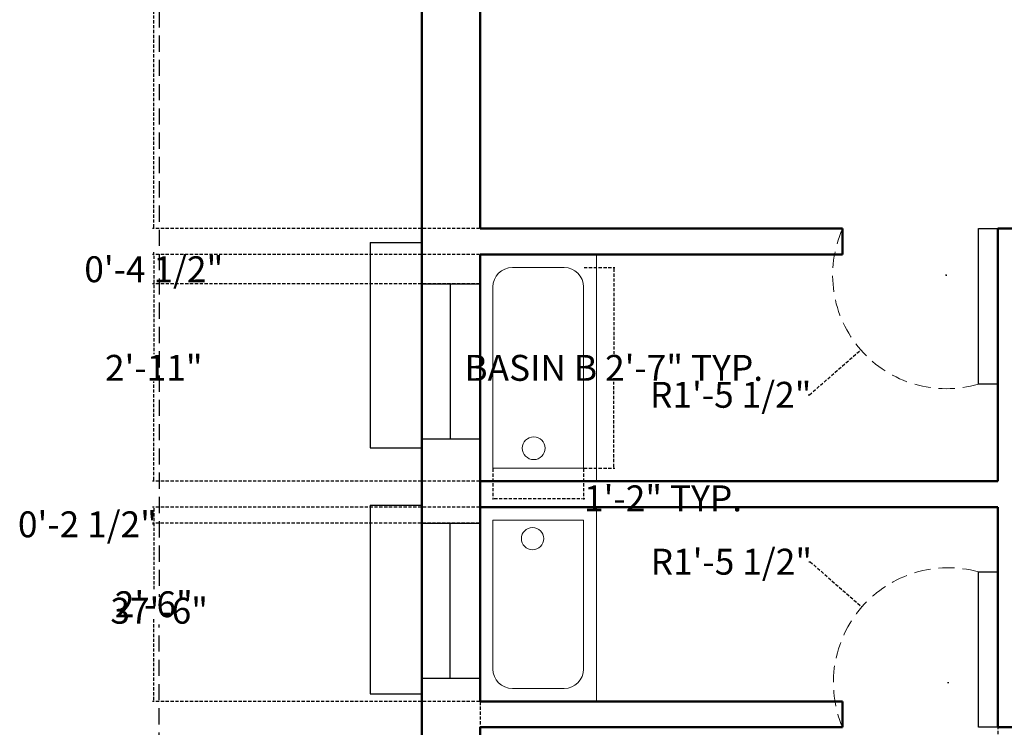
# Model space of a CAD drawing. Units: inches. Extents: x 513 to 1142, y 396 to 927.
# Tile 3 of 31: x 513 to 665, y 637 to 746. Entities that reach past the tile are written whole.
import ezdxf

# ---------------------------------------------------------------- set-up
doc = ezdxf.new("R2010")
doc.units = ezdxf.units.IN
doc.header["$MEASUREMENT"] = 0
doc.linetypes.add('DASHED', pattern=[0.75, 0.5, -0.25])
for name, color, linetype, lineweight in [('A-ANNO-DIMS', 2, 'DASHED', 18), ('A-DOOR', 4, 'Continuous', 25), ('A-DOOR-SWNG', 4, 'DASHED', 13), ('A-FLOR-FIXT', 92, 'Continuous', 18), ('A-WALL', 7, 'Continuous', 50), ('windows', 172, 'Continuous', 25)]:
    doc.layers.add(name, color=color, linetype=linetype, lineweight=lineweight)
doc.styles.get("Standard").update_dxf_attribs({"font": 'arial.ttf'})
doc.dimstyles.get("Standard").update_dxf_attribs({"dimtxt": 4, "dimasz": 0.18, "dimexe": 0.18, "dimexo": 0.0625, "dimgap": 0.09, "dimtad": 0, "dimtih": 1, "dimtoh": 1, "dimdec": 0, "dimrnd": 6, "dimzin": 0, "dimdsep": 46, "dimlunit": 3, "dimtxsty": 'Standard', "dimcen": 0.09, "dimadec": 0, "dimazin": 0, "dimtfac": 1, "dimtdec": 0, "dimtofl": 0, "dimtmove": 0, "dimatfit": 3, "dimfxl": 1, "dimtolj": 1, "dimtzin": 0, "dimarcsym": 0})

# ---------------------------------------------------------------- blocks, each defined once
blk = doc.blocks.new('*D104')
at = {"layer": 'A-ANNO-DIMS', "color": 0, "lineweight": -2, "ltscale": 5, "transparency": 16777216}
for p, q in [((574.93, 879.16), (534.25, 879.16)), ((534.43, 878.98), (534.43, 657.29)), ((534.43, 431.34), (534.43, 653.02)), ((574.93, 431.16), (534.25, 431.16))]:
    blk.add_line(p, q, dxfattribs=at)
at = {"layer": 'A-ANNO-DIMS', "color": 0, "ltscale": 5, "transparency": 16777216}
for points in [[(534.4, 878.98), (534.46, 878.98), (534.43, 879.16)], [(534.4, 431.34), (534.46, 431.34), (534.43, 431.16)]]:
    blk.add_solid(points, dxfattribs=at)
at = {"layer": 'Defpoints', "color": 0, "ltscale": 5, "transparency": 16777216}
for p in [(575, 879.16), (534.43, 431.16), (575, 431.16)]:
    blk.add_point(p, dxfattribs=at)
at = {"layer": 'A-ANNO-DIMS', "color": 0, "ltscale": 5, "transparency": 16777216, "insert": (534.43, 655.16), "char_height": 4, "attachment_point": 5}
blk.add_mtext('\\A1;37\'-6"', dxfattribs=at)
blk = doc.blocks.new('WIN-24IN')
blk.add_line((0, 4.39), (24, 4.39))
blk.add_lwpolyline([(24, 0), (0, 0), (0, 9), (24, 9)], close=True)
blk = doc.blocks.new('DOOR-LEAF-24IN')
blk.add_lwpolyline([(3, 24), (3, 0), (0, 0), (0, 24)], close=True)
blk = doc.blocks.new('BASIN-BOWL-14X26')
for p, q in [((0, 3), (0, 26)), ((0, 26), (14, 26)), ((14, 3), (14, 26)), ((3, 0), (11, 0))]:
    blk.add_line(p, q)
for centre, start, end in [((3, 3), 180, 270), ((11, 3), 270, 0)]:
    blk.add_arc(centre, 3, start, end)
blk = doc.blocks.new('BASIN-BOWL-14X31')
for p, q in [((11, 31), (3, 31)), ((0, 0), (0, 28)), ((14, 0), (14, 28)), ((0, 0), (14, 0))]:
    blk.add_line(p, q)
for centre, start, end in [((3, 28), 90, 180), ((11, 28), 0, 90)]:
    blk.add_arc(centre, 3, start, end)
blk = doc.blocks.new('*D133')
at = {"layer": 'A-ANNO-DIMS', "color": 0, "lineweight": -2, "transparency": 16777216}
for p, q in [((600.06, 708.16), (604.83, 708.16)), ((604.65, 707.98), (604.65, 694.82)), ((604.65, 677.34), (604.65, 690.5)), ((600.06, 677.16), (604.83, 677.16))]:
    blk.add_line(p, q, dxfattribs=at)
at = {"layer": 'A-ANNO-DIMS', "color": 0, "transparency": 16777216}
for points in [[(604.62, 707.98), (604.68, 707.98), (604.65, 708.16)], [(604.62, 677.34), (604.68, 677.34), (604.65, 677.16)]]:
    blk.add_solid(points, dxfattribs=at)
at = {"layer": 'Defpoints', "color": 0, "transparency": 16777216}
for p in [(600, 708.16), (604.65, 708.16), (600, 677.16)]:
    blk.add_point(p, dxfattribs=at)
at = {"layer": 'A-ANNO-DIMS', "color": 0, "transparency": 16777216, "insert": (604.65, 692.66), "char_height": 4, "attachment_point": 5}
blk.add_mtext('\\A1;BASIN B 2\'-7" TYP.', dxfattribs=at)
blk = doc.blocks.new('*D134')
at = {"layer": 'A-ANNO-DIMS', "color": 0, "lineweight": -2, "transparency": 16777216}
for p, q in [((586, 677.1), (586, 672.33)), ((600, 677.1), (600, 672.33)), ((586.18, 672.51), (599.82, 672.51)), ((600, 672.51), (600.18, 672.51))]:
    blk.add_line(p, q, dxfattribs=at)
at = {"layer": 'A-ANNO-DIMS', "color": 0, "transparency": 16777216}
for points in [[(586.18, 672.54), (586.18, 672.48), (586, 672.51)], [(599.82, 672.54), (599.82, 672.48), (600, 672.51)]]:
    blk.add_solid(points, dxfattribs=at)
at = {"layer": 'Defpoints', "color": 0, "transparency": 16777216}
for p in [(586, 677.16), (600, 677.16), (600, 672.51)]:
    blk.add_point(p, dxfattribs=at)
at = {"layer": 'A-ANNO-DIMS', "color": 0, "transparency": 16777216, "insert": (612.27, 672.51), "char_height": 4, "attachment_point": 5}
blk.add_mtext('\\A1;1\'-2" TYP.', dxfattribs=at)
blk = doc.blocks.new('*D139')
at = {"layer": 'A-ANNO-DIMS', "color": 0, "lineweight": -2, "transparency": 16777216}
for p, q in [((583.93, 870.16), (533.42, 870.16)), ((533.6, 869.98), (533.6, 794.29)), ((533.6, 714.34), (533.6, 790.02)), ((583.93, 714.16), (533.42, 714.16))]:
    blk.add_line(p, q, dxfattribs=at)
at = {"layer": 'A-ANNO-DIMS', "color": 0, "transparency": 16777216}
for points in [[(533.57, 869.98), (533.63, 869.98), (533.6, 870.16)], [(533.57, 714.34), (533.63, 714.34), (533.6, 714.16)]]:
    blk.add_solid(points, dxfattribs=at)
at = {"layer": 'Defpoints', "color": 0, "transparency": 16777216}
for p in [(533.6, 870.16), (584, 870.16), (584, 714.16)]:
    blk.add_point(p, dxfattribs=at)
at = {"layer": 'A-ANNO-DIMS', "color": 0, "transparency": 16777216, "insert": (533.6, 792.16), "char_height": 4, "attachment_point": 5}
blk.add_mtext('\\A1;13\'-0"', dxfattribs=at)
blk = doc.blocks.new('*D140')
at = {"layer": 'A-ANNO-DIMS', "color": 0, "lineweight": -2, "transparency": 16777216}
for p, q in [((583.93, 710.16), (533.42, 710.16)), ((533.6, 709.98), (533.6, 694.76)), ((533.6, 675.34), (533.6, 690.56)), ((583.93, 675.16), (533.42, 675.16))]:
    blk.add_line(p, q, dxfattribs=at)
at = {"layer": 'A-ANNO-DIMS', "color": 0, "transparency": 16777216}
for points in [[(533.57, 709.98), (533.63, 709.98), (533.6, 710.16)], [(533.57, 675.34), (533.63, 675.34), (533.6, 675.16)]]:
    blk.add_solid(points, dxfattribs=at)
at = {"layer": 'Defpoints', "color": 0, "transparency": 16777216}
for p in [(533.6, 710.16), (584, 710.16), (584, 675.16)]:
    blk.add_point(p, dxfattribs=at)
at = {"layer": 'A-ANNO-DIMS', "color": 0, "transparency": 16777216, "insert": (533.6, 692.66), "char_height": 4, "attachment_point": 5}
blk.add_mtext('\\A1;2\'-11"', dxfattribs=at)
blk = doc.blocks.new('*D141')
at = {"layer": 'A-ANNO-DIMS', "color": 0, "lineweight": -2, "transparency": 16777216}
for p, q in [((583.93, 671.16), (533.42, 671.16)), ((533.6, 670.98), (533.6, 658.29)), ((533.6, 641.34), (533.6, 654.03)), ((583.93, 641.16), (533.42, 641.16))]:
    blk.add_line(p, q, dxfattribs=at)
at = {"layer": 'A-ANNO-DIMS', "color": 0, "transparency": 16777216}
for points in [[(533.57, 670.98), (533.63, 670.98), (533.6, 671.16)], [(533.57, 641.34), (533.63, 641.34), (533.6, 641.16)]]:
    blk.add_solid(points, dxfattribs=at)
at = {"layer": 'Defpoints', "color": 0, "transparency": 16777216}
for p in [(533.6, 671.16), (584, 671.16), (584, 641.16)]:
    blk.add_point(p, dxfattribs=at)
at = {"layer": 'A-ANNO-DIMS', "color": 0, "transparency": 16777216, "insert": (533.6, 656.16), "char_height": 4, "attachment_point": 5}
blk.add_mtext('\\A1;2\'-6"', dxfattribs=at)
blk = doc.blocks.new('*D147')
at = {"layer": 'A-ANNO-DIMS', "color": 0, "lineweight": -2, "transparency": 16777216}
for p, q in [((584, 671.1), (584, 401.58)), ((664, 671.1), (664, 401.58)), ((584.18, 401.76), (618.58, 401.76)), ((663.82, 401.76), (629.41, 401.76))]:
    blk.add_line(p, q, dxfattribs=at)
at = {"layer": 'A-ANNO-DIMS', "color": 0, "transparency": 16777216}
for points in [[(584.18, 401.79), (584.18, 401.73), (584, 401.76)], [(663.82, 401.79), (663.82, 401.73), (664, 401.76)]]:
    blk.add_solid(points, dxfattribs=at)
at = {"layer": 'Defpoints', "color": 0, "transparency": 16777216}
for p in [(584, 671.16), (664, 671.16), (664, 401.76)]:
    blk.add_point(p, dxfattribs=at)
at = {"layer": 'A-ANNO-DIMS', "color": 0, "transparency": 16777216, "insert": (624, 401.76), "char_height": 4, "attachment_point": 5}
blk.add_mtext('\\A1;6\'-8"', dxfattribs=at)
blk = doc.blocks.new('*D163')
at = {"layer": 'A-ANNO-DIMS', "color": 0, "lineweight": -2, "transparency": 16777216}
for p, q in [((533.6, 710.34), (533.6, 710.52)), ((583.93, 710.16), (533.42, 710.16)), ((583.94, 705.63), (533.42, 705.63)), ((533.6, 705.45), (533.6, 705.27))]:
    blk.add_line(p, q, dxfattribs=at)
at = {"layer": 'A-ANNO-DIMS', "color": 0, "transparency": 16777216}
for points in [[(533.57, 710.34), (533.63, 710.34), (533.6, 710.16)], [(533.57, 705.45), (533.63, 705.45), (533.6, 705.63)]]:
    blk.add_solid(points, dxfattribs=at)
at = {"layer": 'Defpoints', "color": 0, "transparency": 16777216}
for p in [(584, 710.16), (533.6, 705.63), (584.01, 705.63)]:
    blk.add_point(p, dxfattribs=at)
at = {"layer": 'A-ANNO-DIMS', "color": 0, "transparency": 16777216, "insert": (533.6, 707.89), "char_height": 4, "attachment_point": 5}
blk.add_mtext('\\A1;0\'-4 1/2"', dxfattribs=at)
blk = doc.blocks.new('*D164')
at = {"layer": 'A-ANNO-DIMS', "color": 0, "lineweight": -2, "transparency": 16777216}
for p, q in [((583.93, 671.16), (533.42, 671.16)), ((533.6, 670.98), (533.6, 668.86)), ((583.89, 668.68), (533.42, 668.68)), ((533.6, 668.5), (533.42, 668.5)), ((533.6, 668.68), (533.6, 668.5))]:
    blk.add_line(p, q, dxfattribs=at)
at = {"layer": 'A-ANNO-DIMS', "color": 0, "transparency": 16777216}
for points in [[(533.57, 670.98), (533.63, 670.98), (533.6, 671.16)], [(533.57, 668.86), (533.63, 668.86), (533.6, 668.68)]]:
    blk.add_solid(points, dxfattribs=at)
at = {"layer": 'Defpoints', "color": 0, "transparency": 16777216}
for p in [(584, 671.16), (533.6, 668.68), (583.95, 668.68)]:
    blk.add_point(p, dxfattribs=at)
at = {"layer": 'A-ANNO-DIMS', "color": 0, "transparency": 16777216, "insert": (523.35, 668.5), "char_height": 4, "attachment_point": 5}
blk.add_mtext('\\A1;0\'-2 1/2"', dxfattribs=at)
blk = doc.blocks.new('*D187')
at = {"layer": 'A-ANNO-DIMS', "color": 0, "lineweight": -2, "transparency": 16777216}
for p, q in [((634.8, 662.73), (634.98, 662.73)), ((634.98, 662.73), (642.85, 655.85)), ((656.23, 644.06), (656.41, 644.06)), ((656.32, 643.97), (656.32, 644.15))]:
    blk.add_line(p, q, dxfattribs=at)
at = {"layer": 'A-ANNO-DIMS', "color": 0, "transparency": 16777216}
blk.add_solid([(642.87, 655.87), (642.83, 655.83), (642.98, 655.73)], dxfattribs=at)
at = {"layer": 'Defpoints', "color": 0, "transparency": 16777216}
for p in [(642.98, 655.73), (656.32, 644.06)]:
    blk.add_point(p, dxfattribs=at)
at = {"layer": 'A-ANNO-DIMS', "color": 0, "transparency": 16777216, "insert": (622.82, 662.73), "char_height": 4, "attachment_point": 5}
blk.add_mtext('\\A1;R1\'-5 1/2"', dxfattribs=at)
blk = doc.blocks.new('*D188')
at = {"layer": 'A-ANNO-DIMS', "color": 0, "lineweight": -2, "transparency": 16777216}
for p, q in [((655.93, 706.99), (656.11, 706.99)), ((656.02, 706.9), (656.02, 707.08)), ((634.88, 688.5), (642.67, 695.32)), ((634.7, 688.5), (634.88, 688.5))]:
    blk.add_line(p, q, dxfattribs=at)
at = {"layer": 'A-ANNO-DIMS', "color": 0, "transparency": 16777216}
blk.add_solid([(642.65, 695.34), (642.69, 695.29), (642.81, 695.43)], dxfattribs=at)
at = {"layer": 'Defpoints', "color": 0, "transparency": 16777216}
for p in [(656.02, 706.99), (642.81, 695.43)]:
    blk.add_point(p, dxfattribs=at)
at = {"layer": 'A-ANNO-DIMS', "color": 0, "transparency": 16777216, "insert": (622.72, 688.5), "char_height": 4, "attachment_point": 5}
blk.add_mtext('\\A1;R1\'-5 1/2"', dxfattribs=at)

msp = doc.modelspace()

# ---------------------------------------------------------------- linework, layer by layer
at = {"layer": 'A-DOOR-SWNG', "ltscale": 5}
for centre, radius, start, end in [((656.02, 706.99), 17.55, 155.9122, 286.4597), ((656.32, 644.06), 17.73, 74.72, 202.9082)]:
    msp.add_arc(centre, radius, start, end, dxfattribs=at)
at = {"layer": 'A-FLOR-FIXT'}
for p, q in [((602, 710.16), (602, 675.16)), ((602, 671.16), (602, 641.16))]:
    msp.add_line(p, q, dxfattribs=at)
for centre, radius in [((592.29, 680.26), 1.76), ((592.11, 666.29), 1.72)]:
    msp.add_circle(centre, radius, dxfattribs=at)
at = {"layer": 'A-WALL'}
for p, q in [((575, 879.16), (575, 431.16)), ((584, 870.16), (584, 714.16)), ((640, 714.16), (584, 714.16)), ((640, 714.16), (640, 710.16)), ((704, 714.16), (664, 714.16)), ((664, 714.16), (664, 675.16)), ((640, 710.16), (584, 710.16)), ((584, 710.16), (584, 641.16)), ((584, 675.16), (664, 675.16)), ((584, 671.16), (664, 671.16)), ((664, 671.16), (664, 637.16)), ((584, 641.16), (640, 641.16)), ((640, 641.16), (640, 637.16)), ((584, 637.16), (640, 637.16)), ((584, 637.16), (584, 497.16)), ((664, 637.16), (716, 637.16))]:
    msp.add_line(p, q, dxfattribs=at)
at = {"layer": 'windows'}
for p, q in [((567, 712), (575, 712)), ((567, 712), (567, 680.32)), ((567, 680.32), (575, 680.32)), ((567, 671.47), (575, 671.47)), ((567, 671.47), (567, 642.34)), ((567, 642.34), (575, 642.34))]:
    msp.add_line(p, q, dxfattribs=at)

# ---------------------------------------------------------------- block references
at = {"layer": 'A-DOOR', "rotation": 180}
msp.add_blockref('DOOR-LEAF-24IN', (664, 714.16), dxfattribs=at)
at = {"layer": 'A-DOOR'}
msp.add_blockref('DOOR-LEAF-24IN', (661, 637.16), dxfattribs=at)
at = {"layer": 'A-FLOR-FIXT'}
for name, p in [('BASIN-BOWL-14X31', (585.99, 677.16)), ('BASIN-BOWL-14X26', (585.99, 643.16))]:
    msp.add_blockref(name, p, dxfattribs=at)
at = {"layer": 'windows', "rotation": 270.0000000000002}
for p in [(575.01, 705.63), (574.95, 668.68)]:
    msp.add_blockref('WIN-24IN', p, dxfattribs=at)

# ---------------------------------------------------------------- dimensions: what is measured, and where the dimension line sits
at = {"layer": 'A-ANNO-DIMS', "ltscale": 5}
dim = msp.add_linear_dim(base=(534.43, 431.16), p1=(575, 879.16), p2=(575, 431.16), angle=90, dimstyle='Standard', override={"dimclrd": 0, "dimclre": 0, "dimclrt": 0}, dxfattribs=at)
dim.commit()
dim.dimension.update_dxf_attribs({"geometry": '*D104', "text_midpoint": (534.43, 655.16)})
at = {"layer": 'A-ANNO-DIMS'}
for base, p1, p2, picture, middle in [((533.6, 870.16), (584, 714.16), (584, 870.16), '*D139', (533.6, 792.16)), ((533.6, 705.63), (584, 710.16), (584.01, 705.63), '*D163', (533.6, 707.89)), ((533.6, 710.16), (584, 675.16), (584, 710.16), '*D140', (533.6, 692.66)), ((533.6, 668.68), (584, 671.16), (583.95, 668.68), '*D164', (523.35, 668.5)), ((533.6, 671.16), (584, 641.16), (584, 671.16), '*D141', (533.6, 656.16))]:
    dim = msp.add_linear_dim(base=base, p1=p1, p2=p2, angle=90, dimstyle='Standard', override={"dimdec": 1, "dimlfac": 1, "dimrnd": 0, "dimzin": 1, "dimdsep": 46, "dimlunit": 4, "dimfrac": 2}, dxfattribs=at)
    dim.commit()
    dim.dimension.update_dxf_attribs({"geometry": picture, "text_midpoint": middle})
dim = msp.add_linear_dim(base=(604.65, 708.16), p1=(600, 677.16), p2=(600, 708.16), angle=90, text='BASIN B <> TYP.', dimstyle='Standard', override={"dimdec": 1, "dimlfac": 1, "dimrnd": 0, "dimzin": 1, "dimdsep": 46, "dimlunit": 4, "dimfrac": 2}, dxfattribs=at)
dim.commit()
dim.dimension.update_dxf_attribs({"geometry": '*D133', "text_midpoint": (604.65, 692.66)})
for center, mpoint, picture, middle in [((656.02, 706.99), (642.81, 695.43), '*D188', (622.72, 688.5)), ((656.32, 644.06), (642.98, 655.73), '*D187', (622.82, 662.73))]:
    dim = msp.add_radius_dim(center=center, mpoint=mpoint, dimstyle='Standard', override={"dimdec": 1, "dimlfac": 1, "dimrnd": 0, "dimzin": 1, "dimdsep": 46, "dimlunit": 4, "dimfrac": 2}, dxfattribs=at)
    dim.commit()
    dim.dimension.update_dxf_attribs({"geometry": picture, "text_midpoint": middle, "dimtype": 164})
dim = msp.add_linear_dim(base=(600, 672.51), p1=(586, 677.16), p2=(600, 677.16), text='<> TYP.', dimstyle='Standard', override={"dimdec": 1, "dimlfac": 1, "dimrnd": 0, "dimzin": 1, "dimdsep": 46, "dimlunit": 4, "dimfrac": 2}, dxfattribs=at)
dim.commit()
dim.dimension.update_dxf_attribs({"geometry": '*D134', "text_midpoint": (612.27, 672.51)})
dim = msp.add_linear_dim(base=(664, 401.76), p1=(584, 671.16), p2=(664, 671.16), dimstyle='Standard', override={"dimdec": 1, "dimlfac": 1, "dimrnd": 0, "dimzin": 1, "dimdsep": 46, "dimlunit": 4, "dimfrac": 2}, dxfattribs=at)
dim.commit()
dim.dimension.update_dxf_attribs({"geometry": '*D147', "text_midpoint": (624, 401.76)})

doc.saveas('drawing.dxf')
